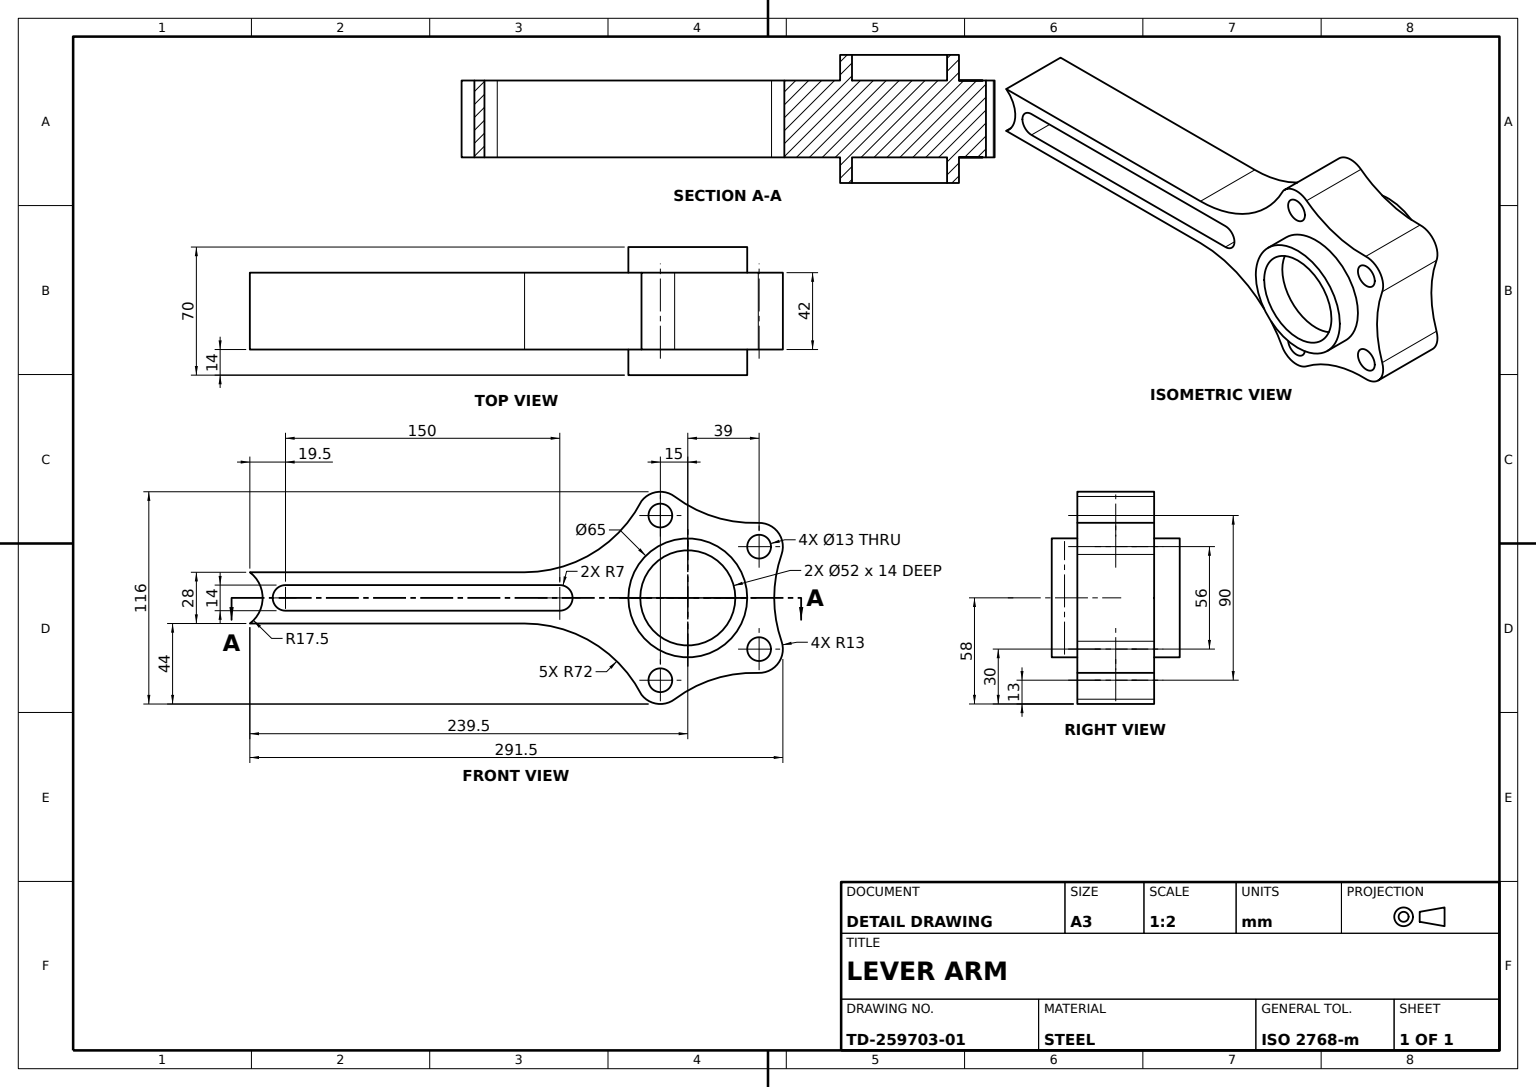
from build123d import *

# Parameters (mm, degrees)
HUB_BLOCK_SKETCH_R   = 32.5
HUB_BLOCK_SKETCH_R_2 = 26
HUB_BLOCK_DEPTH      = 35
ARM_PROFILE_SKETCH_R = 6.5
ARM_BODY_DEPTH       = 42


with BuildPart() as part:
    # Hub Block Sketch → Hub Block (new, symmetric)
    with BuildSketch(Plane.XY):
        Circle(HUB_BLOCK_SKETCH_R)
        Circle(HUB_BLOCK_SKETCH_R_2, mode=Mode.SUBTRACT)
    extrude(amount=HUB_BLOCK_DEPTH, both=True)

    # Arm Profile Sketch → Arm Body (add)
    with BuildSketch(Plane(origin=(0, 0, -21), x_dir=(-1, 0, 0), z_dir=(0, 0, -1))):
        with BuildLine():
            ThreePointArc((89.262059242, -14), (51.834907578, -24.492209287), (25.315908922, -52.910880046))
            ThreePointArc((25.315908922, -52.910880046), (16.763184773, -57.879874978), (7.189691393, -55.392260556))
            ThreePointArc((7.189691393, -55.392260556), (-14.44681941, -44.272249892), (-38.551485077, -40.992260556))
            ThreePointArc((-38.551485077, -40.992260556), (-49.467382276, -35.70933903), (-51.274422727, -23.717647059))
            ThreePointArc((-51.274422727, -23.717647059), (-47.255840909, 0), (-51.274422727, 23.717647059))
            ThreePointArc((-51.274422727, 23.717647059), (-49.467382276, 35.70933903), (-38.551485077, 40.992260556))
            ThreePointArc((-38.551485077, 40.992260556), (-14.44681941, 44.272249892), (7.189691393, 55.392260556))
            ThreePointArc((7.189691393, 55.392260556), (16.763184773, 57.879874978), (25.315908922, 52.910880046))
            ThreePointArc((25.315908922, 52.910880046), (51.834907578, 24.492209287), (89.262059242, 14))
            Line((89.262059242, 14), (239.5, 14))
            ThreePointArc((239.5, 14), (232.5, 0), (239.5, -14))
            Line((239.5, -14), (89.262059242, -14))
        make_face()
        with Locations((15, -45)):
            Circle(ARM_PROFILE_SKETCH_R, mode=Mode.SUBTRACT)
        with Locations((15, 45)):
            Circle(ARM_PROFILE_SKETCH_R, mode=Mode.SUBTRACT)
        with Locations((-39, -28)):
            Circle(ARM_PROFILE_SKETCH_R, mode=Mode.SUBTRACT)
        with Locations((-39, 28)):
            Circle(ARM_PROFILE_SKETCH_R, mode=Mode.SUBTRACT)
        with BuildLine():
            ThreePointArc((220, -7), (227, 0), (220, 7))
            Line((220, 7), (70, 7))
            ThreePointArc((70, 7), (63, 0), (70, -7))
            Line((70, -7), (220, -7))
        make_face(mode=Mode.SUBTRACT)
    extrude(amount=-ARM_BODY_DEPTH)


solid = part.part
